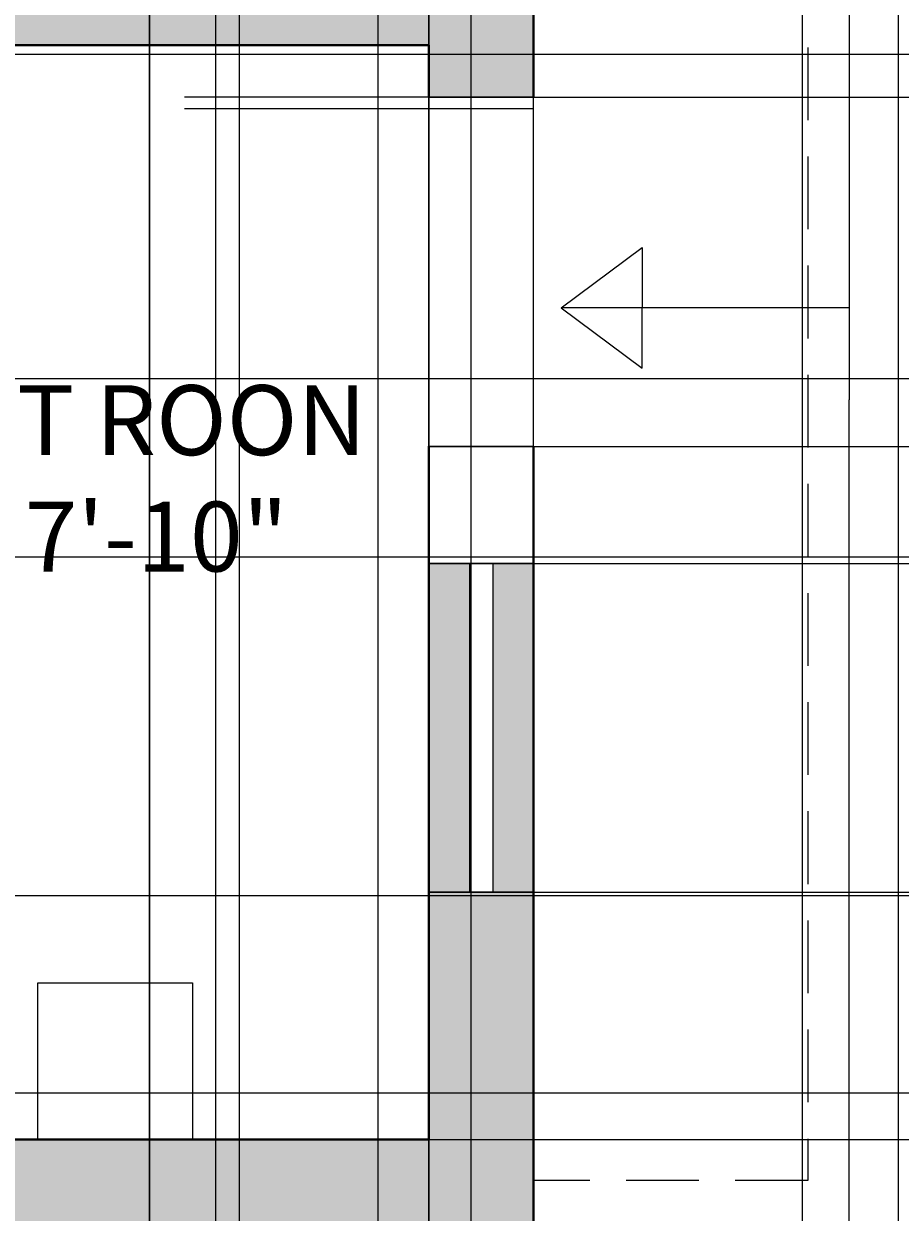
# Model space of a CAD drawing. Units: inches. Extents: x 818 to 1898, y 976 to 2364.
# Tile 53 of 96: x 1671 to 1746, y 1690 to 1792. Entities that reach past the tile are written whole.
import ezdxf

# ---------------------------------------------------------------- set-up
doc = ezdxf.new("R2010")
doc.units = ezdxf.units.IN
doc.header["$LTSCALE"] = 5
doc.header["$MEASUREMENT"] = 0
doc.linetypes.add('HIDDEN', pattern=[0.375, 0.25, -0.125])
for name, color, linetype, lineweight in [('A-ANNO-DIMS', 2, 'Continuous', 18), ('A-ANNO-SYMB', 7, 'Continuous', 18), ('A-AREA-IDEN', 7, 'Continuous', 18), ('A-DOOR', 3, 'Continuous', 25), ('A-FLOR-OVHD', 8, 'HIDDEN', 13), ('A-FLOR-STRS', 7, 'Continuous', 25), ('A-FURN', 8, 'Continuous', 18), ('A-GLAZ', 4, 'Continuous', 18), ('A-WALL', 7, 'Continuous', 40)]:
    doc.layers.add(name, color=color, linetype=linetype, lineweight=lineweight)
doc.layers.add('A-GLAZ-PATT', color=141, linetype='Continuous', lineweight=9, true_color=0xadddf7)
doc.layers.add('A-WALL-PATT', color=251, linetype='Continuous', lineweight=13, true_color=0x636466)
doc.styles.get("Standard").update_dxf_attribs({"font": 'arial.ttf'})
doc.dimstyles.get("Standard").update_dxf_attribs({"dimtxt": 0.18, "dimasz": 0.18, "dimexe": 0.18, "dimexo": 0.0625, "dimgap": 0.09, "dimtad": 0, "dimtih": 1, "dimtoh": 1, "dimdec": 4, "dimzin": 0, "dimdsep": 46, "dimtxsty": 'Standard', "dimcen": 0.09, "dimadec": 0, "dimazin": 0, "dimtfac": 1, "dimtdec": 4, "dimtofl": 0, "dimtmove": 0, "dimatfit": 3, "dimfxl": 1, "dimtolj": 1, "dimtzin": 0, "dimarcsym": 0})

# ---------------------------------------------------------------- blocks, each defined once
blk = doc.blocks.new('ARROW-STEP-UP')
at = {"ltscale": 5}
for p, q in [((0, 5.17), (6.97, 10.34)), ((6.97, 10.34), (6.97, 5.17)), ((24.75, 5.17), (0, 5.17)), ((0, 5.17), (6.97, 0)), ((6.97, 0), (6.97, 5.17))]:
    blk.add_line(p, q, dxfattribs=at)
blk = doc.blocks.new('*D71')
at = {"layer": 'A-ANNO-DIMS', "color": 0, "lineweight": -2, "ltscale": 5, "transparency": 16777216}
for p, q in [((1714.79, 2053.08), (1897.92, 2053.08)), ((1897.74, 2052.9), (1897.74, 1699.76)), ((1897.74, 1346.26), (1897.74, 1699.4)), ((1714.79, 1346.08), (1897.92, 1346.08))]:
    blk.add_line(p, q, dxfattribs=at)
at = {"layer": 'A-ANNO-DIMS', "color": 0, "ltscale": 5, "transparency": 16777216}
for points in [[(1897.71, 2052.9), (1897.77, 2052.9), (1897.74, 2053.08)], [(1897.71, 1346.26), (1897.77, 1346.26), (1897.74, 1346.08)]]:
    blk.add_solid(points, dxfattribs=at)
at = {"layer": 'Defpoints', "color": 0, "ltscale": 5, "transparency": 16777216}
for p in [(1714.73, 2053.08), (1897.74, 2053.08), (1714.73, 1346.08)]:
    blk.add_point(p, dxfattribs=at)
at = {"layer": 'A-ANNO-DIMS', "color": 0, "ltscale": 5, "transparency": 16777216, "insert": (1897.74, 1699.58), "char_height": 0.18, "attachment_point": 5}
blk.add_mtext('\\A1;707', dxfattribs=at)
blk = doc.blocks.new('*D75')
at = {"layer": 'A-ANNO-DIMS', "color": 0, "lineweight": -2, "ltscale": 5, "transparency": 16777216}
for p, q in [((1705.79, 1785.61), (1897.92, 1785.61)), ((1897.74, 1785.43), (1897.74, 1770.79)), ((1897.74, 1755.79), (1897.74, 1770.43)), ((1705.79, 1755.61), (1897.92, 1755.61))]:
    blk.add_line(p, q, dxfattribs=at)
at = {"layer": 'A-ANNO-DIMS', "color": 0, "ltscale": 5, "transparency": 16777216}
for points in [[(1897.71, 1785.43), (1897.77, 1785.43), (1897.74, 1785.61)], [(1897.71, 1755.79), (1897.77, 1755.79), (1897.74, 1755.61)]]:
    blk.add_solid(points, dxfattribs=at)
at = {"layer": 'Defpoints', "color": 0, "ltscale": 5, "transparency": 16777216}
for p in [(1705.73, 1785.61), (1705.73, 1755.61), (1897.74, 1755.61)]:
    blk.add_point(p, dxfattribs=at)
at = {"layer": 'A-ANNO-DIMS', "color": 0, "ltscale": 5, "transparency": 16777216, "insert": (1897.74, 1770.61), "char_height": 0.18, "attachment_point": 5}
blk.add_mtext('\\A1;30', dxfattribs=at)
blk = doc.blocks.new('*D85')
at = {"layer": 'A-ANNO-DIMS', "color": 0, "lineweight": -2, "ltscale": 5, "transparency": 16777216}
for p, q in [((1258.79, 2053.08), (1897.92, 2053.08)), ((1897.74, 2052.9), (1897.74, 1876.76)), ((1897.74, 1700.26), (1897.74, 1876.4)), ((1258.79, 1700.08), (1897.92, 1700.08))]:
    blk.add_line(p, q, dxfattribs=at)
at = {"layer": 'A-ANNO-DIMS', "color": 0, "ltscale": 5, "transparency": 16777216}
for points in [[(1897.71, 2052.9), (1897.77, 2052.9), (1897.74, 2053.08)], [(1897.71, 1700.26), (1897.77, 1700.26), (1897.74, 1700.08)]]:
    blk.add_solid(points, dxfattribs=at)
at = {"layer": 'Defpoints', "color": 0, "ltscale": 5, "transparency": 16777216}
for p in [(1258.73, 2053.08), (1897.74, 2053.08), (1258.73, 1700.08)]:
    blk.add_point(p, dxfattribs=at)
at = {"layer": 'A-ANNO-DIMS', "color": 0, "ltscale": 5, "transparency": 16777216, "insert": (1897.74, 1876.58), "char_height": 0.18, "attachment_point": 5}
blk.add_mtext('\\A1;353', dxfattribs=at)
blk = doc.blocks.new('*D103')
at = {"layer": 'A-ANNO-DIMS', "color": 0, "lineweight": -2, "ltscale": 5, "transparency": 16777216}
for p, q in [((1626.57, 1071.12), (1626.57, 2363.87)), ((1626.75, 2363.69), (1657.7, 2363.69)), ((1689.29, 2363.69), (1658.35, 2363.69)), ((1689.47, 1071.12), (1689.47, 2363.87))]:
    blk.add_line(p, q, dxfattribs=at)
at = {"layer": 'A-ANNO-DIMS', "color": 0, "ltscale": 5, "transparency": 16777216}
for points in [[(1626.75, 2363.72), (1626.75, 2363.66), (1626.57, 2363.69)], [(1689.29, 2363.72), (1689.29, 2363.66), (1689.47, 2363.69)]]:
    blk.add_solid(points, dxfattribs=at)
at = {"layer": 'Defpoints', "color": 0, "ltscale": 5, "transparency": 16777216}
for p in [(1689.47, 2363.69), (1626.57, 1071.06), (1689.47, 1071.06)]:
    blk.add_point(p, dxfattribs=at)
at = {"layer": 'A-ANNO-DIMS', "color": 0, "ltscale": 5, "transparency": 16777216, "insert": (1658.02, 2363.69), "char_height": 0.18, "attachment_point": 5}
blk.add_mtext('\\A1;62.9', dxfattribs=at)
blk = doc.blocks.new('*D104')
at = {"layer": 'A-ANNO-DIMS', "color": 0, "lineweight": -2, "ltscale": 5, "transparency": 16777216}
for p, q in [((1689.47, 1071.12), (1689.47, 2363.87)), ((1689.65, 2363.69), (1717.4, 2363.69)), ((1745.9, 2363.69), (1718.15, 2363.69)), ((1746.08, 1071.12), (1746.08, 2363.87))]:
    blk.add_line(p, q, dxfattribs=at)
at = {"layer": 'A-ANNO-DIMS', "color": 0, "ltscale": 5, "transparency": 16777216}
for points in [[(1689.65, 2363.72), (1689.65, 2363.66), (1689.47, 2363.69)], [(1745.9, 2363.72), (1745.9, 2363.66), (1746.08, 2363.69)]]:
    blk.add_solid(points, dxfattribs=at)
at = {"layer": 'Defpoints', "color": 0, "ltscale": 5, "transparency": 16777216}
for p in [(1746.08, 2363.69), (1689.47, 1071.06), (1746.08, 1071.06)]:
    blk.add_point(p, dxfattribs=at)
at = {"layer": 'A-ANNO-DIMS', "color": 0, "ltscale": 5, "transparency": 16777216, "insert": (1717.78, 2363.69), "char_height": 0.18, "attachment_point": 5}
blk.add_mtext('\\A1;56.61', dxfattribs=at)
blk = doc.blocks.new('*D119')
at = {"layer": 'A-ANNO-DIMS', "color": 0, "lineweight": -2, "ltscale": 5, "transparency": 16777216}
for p, q in [((1766.29, 1716.99), (818.03, 1716.99)), ((818.21, 1716.81), (818.21, 1672.43)), ((818.21, 1627.69), (818.21, 1672.06)), ((1766.29, 1627.51), (818.03, 1627.51))]:
    blk.add_line(p, q, dxfattribs=at)
at = {"layer": 'A-ANNO-DIMS', "color": 0, "ltscale": 5, "transparency": 16777216}
for points in [[(818.18, 1716.81), (818.24, 1716.81), (818.21, 1716.99)], [(818.18, 1627.69), (818.24, 1627.69), (818.21, 1627.51)]]:
    blk.add_solid(points, dxfattribs=at)
at = {"layer": 'Defpoints', "color": 0, "ltscale": 5, "transparency": 16777216}
for p in [(818.21, 1716.99), (1766.35, 1716.99), (1766.35, 1627.51)]:
    blk.add_point(p, dxfattribs=at)
at = {"layer": 'A-ANNO-DIMS', "color": 0, "ltscale": 5, "transparency": 16777216, "insert": (818.21, 1672.25), "char_height": 0.18, "attachment_point": 5}
blk.add_mtext('\\A1;89.48', dxfattribs=at)
blk = doc.blocks.new('*D120')
at = {"layer": 'A-ANNO-DIMS', "color": 0, "lineweight": -2, "ltscale": 5, "transparency": 16777216}
for p, q in [((1766.29, 1797.72), (818.03, 1797.72)), ((818.21, 1797.54), (818.21, 1757.53)), ((818.21, 1717.17), (818.21, 1757.17)), ((1766.29, 1716.99), (818.03, 1716.99))]:
    blk.add_line(p, q, dxfattribs=at)
at = {"layer": 'A-ANNO-DIMS', "color": 0, "ltscale": 5, "transparency": 16777216}
for points in [[(818.18, 1797.54), (818.24, 1797.54), (818.21, 1797.72)], [(818.18, 1717.17), (818.24, 1717.17), (818.21, 1716.99)]]:
    blk.add_solid(points, dxfattribs=at)
at = {"layer": 'Defpoints', "color": 0, "ltscale": 5, "transparency": 16777216}
for p in [(818.21, 1797.72), (1766.35, 1797.72), (1766.35, 1716.99)]:
    blk.add_point(p, dxfattribs=at)
at = {"layer": 'A-ANNO-DIMS', "color": 0, "ltscale": 5, "transparency": 16777216, "insert": (818.21, 1757.35), "char_height": 0.18, "attachment_point": 5}
blk.add_mtext('\\A1;80.73', dxfattribs=at)
blk = doc.blocks.new('*D154')
at = {"layer": 'A-ANNO-DIMS', "color": 0, "lineweight": -2, "ltscale": 5, "transparency": 16777216}
for p, q in [((1701.37, 1290.14), (1701.37, 2363.87)), ((1701.55, 2363.69), (1705.22, 2363.69)), ((1709.19, 2363.69), (1705.52, 2363.69)), ((1709.37, 1298.14), (1709.37, 2363.87))]:
    blk.add_line(p, q, dxfattribs=at)
at = {"layer": 'A-ANNO-DIMS', "color": 0, "ltscale": 5, "transparency": 16777216}
for points in [[(1701.55, 2363.72), (1701.55, 2363.66), (1701.37, 2363.69)], [(1709.19, 2363.72), (1709.19, 2363.66), (1709.37, 2363.69)]]:
    blk.add_solid(points, dxfattribs=at)
at = {"layer": 'Defpoints', "color": 0, "ltscale": 5, "transparency": 16777216}
for p in [(1709.37, 2363.69), (1709.37, 1298.08), (1701.37, 1290.08)]:
    blk.add_point(p, dxfattribs=at)
at = {"layer": 'A-ANNO-DIMS', "color": 0, "ltscale": 5, "transparency": 16777216, "insert": (1705.37, 2363.69), "char_height": 0.18, "attachment_point": 5}
blk.add_mtext('\\A1;8', dxfattribs=at)
blk = doc.blocks.new('*D186')
at = {"layer": 'A-ANNO-DIMS', "color": 0, "lineweight": -2, "ltscale": 5, "transparency": 16777216}
for p, q in [((1714.73, 1549.14), (1714.73, 2363.87)), ((1714.91, 2363.69), (1725.82, 2363.69)), ((1737.66, 2363.69), (1726.75, 2363.69)), ((1737.84, 1549.14), (1737.84, 2363.87))]:
    blk.add_line(p, q, dxfattribs=at)
at = {"layer": 'A-ANNO-DIMS', "color": 0, "ltscale": 5, "transparency": 16777216}
for points in [[(1714.91, 2363.72), (1714.91, 2363.66), (1714.73, 2363.69)], [(1737.66, 2363.72), (1737.66, 2363.66), (1737.84, 2363.69)]]:
    blk.add_solid(points, dxfattribs=at)
at = {"layer": 'Defpoints', "color": 0, "ltscale": 5, "transparency": 16777216}
for p in [(1737.84, 2363.69), (1714.73, 1549.08), (1737.84, 1549.08)]:
    blk.add_point(p, dxfattribs=at)
at = {"layer": 'A-ANNO-DIMS', "color": 0, "ltscale": 5, "transparency": 16777216, "insert": (1726.28, 2363.69), "char_height": 0.18, "attachment_point": 5}
blk.add_mtext('\\A1;23.116', dxfattribs=at)
blk = doc.blocks.new('*D195')
at = {"layer": 'A-ANNO-DIMS', "color": 0, "lineweight": -2, "ltscale": 5, "transparency": 16777216}
for p, q in [((1681.73, 1379.14), (1681.73, 2363.87)), ((1681.91, 2363.69), (1693.51, 2363.69)), ((1705.55, 2363.69), (1693.95, 2363.69)), ((1705.73, 1355.14), (1705.73, 2363.87))]:
    blk.add_line(p, q, dxfattribs=at)
at = {"layer": 'A-ANNO-DIMS', "color": 0, "ltscale": 5, "transparency": 16777216}
for points in [[(1681.91, 2363.72), (1681.91, 2363.66), (1681.73, 2363.69)], [(1705.55, 2363.72), (1705.55, 2363.66), (1705.73, 2363.69)]]:
    blk.add_solid(points, dxfattribs=at)
at = {"layer": 'Defpoints', "color": 0, "ltscale": 5, "transparency": 16777216}
for p in [(1705.73, 2363.69), (1681.73, 1379.08), (1705.73, 1355.08)]:
    blk.add_point(p, dxfattribs=at)
at = {"layer": 'A-ANNO-DIMS', "color": 0, "ltscale": 5, "transparency": 16777216, "insert": (1693.73, 2363.69), "char_height": 0.18, "attachment_point": 5}
blk.add_mtext('\\A1;24', dxfattribs=at)
blk = doc.blocks.new('*D212')
at = {"layer": 'A-ANNO-DIMS', "color": 0, "lineweight": -2, "ltscale": 5, "transparency": 16777216}
for p, q in [((1681.73, 1900.02), (1681.73, 975.66)), ((1705.73, 1876.02), (1705.73, 975.66)), ((1681.91, 975.84), (1693.51, 975.84)), ((1705.55, 975.84), (1693.95, 975.84))]:
    blk.add_line(p, q, dxfattribs=at)
at = {"layer": 'A-ANNO-DIMS', "color": 0, "ltscale": 5, "transparency": 16777216}
for points in [[(1681.91, 975.87), (1681.91, 975.81), (1681.73, 975.84)], [(1705.55, 975.87), (1705.55, 975.81), (1705.73, 975.84)]]:
    blk.add_solid(points, dxfattribs=at)
at = {"layer": 'Defpoints', "color": 0, "ltscale": 5, "transparency": 16777216}
for p in [(1681.73, 1900.08), (1705.73, 1876.08), (1705.73, 975.84)]:
    blk.add_point(p, dxfattribs=at)
at = {"layer": 'A-ANNO-DIMS', "color": 0, "ltscale": 5, "transparency": 16777216, "insert": (1693.73, 975.84), "char_height": 0.18, "attachment_point": 5}
blk.add_mtext('\\A1;24', dxfattribs=at)
blk = doc.blocks.new('*D216')
at = {"layer": 'A-ANNO-DIMS', "color": 0, "lineweight": -2, "ltscale": 5, "transparency": 16777216}
for p, q in [((1705.79, 1717.32), (1897.92, 1717.32)), ((1897.74, 1717.14), (1897.74, 1706.88)), ((1897.74, 1696.26), (1897.74, 1706.52)), ((1705.79, 1696.08), (1897.92, 1696.08))]:
    blk.add_line(p, q, dxfattribs=at)
at = {"layer": 'A-ANNO-DIMS', "color": 0, "ltscale": 5, "transparency": 16777216}
for points in [[(1897.71, 1717.14), (1897.77, 1717.14), (1897.74, 1717.32)], [(1897.71, 1696.26), (1897.77, 1696.26), (1897.74, 1696.08)]]:
    blk.add_solid(points, dxfattribs=at)
at = {"layer": 'Defpoints', "color": 0, "ltscale": 5, "transparency": 16777216}
for p in [(1705.73, 1717.32), (1897.74, 1717.32), (1705.73, 1696.08)]:
    blk.add_point(p, dxfattribs=at)
at = {"layer": 'A-ANNO-DIMS', "color": 0, "ltscale": 5, "transparency": 16777216, "insert": (1897.74, 1706.7), "char_height": 0.18, "attachment_point": 5}
blk.add_mtext('\\A1;21.24', dxfattribs=at)
blk = doc.blocks.new('*D217')
at = {"layer": 'A-ANNO-DIMS', "color": 0, "lineweight": -2, "ltscale": 5, "transparency": 16777216}
for p, q in [((1705.79, 1745.56), (1897.92, 1745.56)), ((1897.74, 1745.38), (1897.74, 1731.62)), ((1897.74, 1717.5), (1897.74, 1731.26)), ((1705.79, 1717.32), (1897.92, 1717.32))]:
    blk.add_line(p, q, dxfattribs=at)
at = {"layer": 'A-ANNO-DIMS', "color": 0, "ltscale": 5, "transparency": 16777216}
for points in [[(1897.71, 1745.38), (1897.77, 1745.38), (1897.74, 1745.56)], [(1897.71, 1717.5), (1897.77, 1717.5), (1897.74, 1717.32)]]:
    blk.add_solid(points, dxfattribs=at)
at = {"layer": 'Defpoints', "color": 0, "ltscale": 5, "transparency": 16777216}
for p in [(1705.73, 1745.56), (1897.74, 1745.56), (1705.73, 1717.32)]:
    blk.add_point(p, dxfattribs=at)
at = {"layer": 'A-ANNO-DIMS', "color": 0, "ltscale": 5, "transparency": 16777216, "insert": (1897.74, 1731.44), "char_height": 0.18, "attachment_point": 5}
blk.add_mtext('\\A1;28.24', dxfattribs=at)
blk = doc.blocks.new('*D221')
at = {"layer": 'A-ANNO-DIMS', "color": 0, "lineweight": -2, "ltscale": 5, "transparency": 16777216}
for p, q in [((1668.18, 1696.02), (1668.18, 975.66)), ((1705.73, 1696.02), (1705.73, 975.66)), ((1668.36, 975.84), (1686.56, 975.84)), ((1705.55, 975.84), (1687.35, 975.84))]:
    blk.add_line(p, q, dxfattribs=at)
at = {"layer": 'A-ANNO-DIMS', "color": 0, "ltscale": 5, "transparency": 16777216}
for points in [[(1668.36, 975.87), (1668.36, 975.81), (1668.18, 975.84)], [(1705.55, 975.87), (1705.55, 975.81), (1705.73, 975.84)]]:
    blk.add_solid(points, dxfattribs=at)
at = {"layer": 'Defpoints', "color": 0, "ltscale": 5, "transparency": 16777216}
for p in [(1668.18, 1696.08), (1705.73, 1696.08), (1705.73, 975.84)]:
    blk.add_point(p, dxfattribs=at)
at = {"layer": 'A-ANNO-DIMS', "color": 0, "ltscale": 5, "transparency": 16777216, "insert": (1686.95, 975.84), "char_height": 0.18, "attachment_point": 5}
blk.add_mtext('\\A1;37.54', dxfattribs=at)
blk = doc.blocks.new('*D228')
at = {"layer": 'A-ANNO-DIMS', "color": 0, "lineweight": -2, "ltscale": 5, "transparency": 16777216}
for p, q in [((1687.39, 1802.02), (1687.39, 975.66)), ((1705.73, 1802.02), (1705.73, 975.66)), ((1687.57, 975.84), (1696.17, 975.84)), ((1705.55, 975.84), (1696.94, 975.84))]:
    blk.add_line(p, q, dxfattribs=at)
at = {"layer": 'A-ANNO-DIMS', "color": 0, "ltscale": 5, "transparency": 16777216}
for points in [[(1687.57, 975.87), (1687.57, 975.81), (1687.39, 975.84)], [(1705.55, 975.87), (1705.55, 975.81), (1705.73, 975.84)]]:
    blk.add_solid(points, dxfattribs=at)
at = {"layer": 'Defpoints', "color": 0, "ltscale": 5, "transparency": 16777216}
for p in [(1687.39, 1802.08), (1705.73, 1802.08), (1705.73, 975.84)]:
    blk.add_point(p, dxfattribs=at)
at = {"layer": 'A-ANNO-DIMS', "color": 0, "ltscale": 5, "transparency": 16777216, "insert": (1696.56, 975.84), "char_height": 0.18, "attachment_point": 5}
blk.add_mtext('\\A1;18.33', dxfattribs=at)
blk = doc.blocks.new('*D268')
at = {"layer": 'A-ANNO-DIMS', "color": 0, "lineweight": -2, "ltscale": 5, "transparency": 16777216}
for p, q in [((1741.9, 1890.29), (1897.92, 1890.29)), ((1897.74, 1890.11), (1897.74, 1788.87)), ((1897.74, 1687.26), (1897.74, 1788.5)), ((1741.9, 1687.08), (1897.92, 1687.08))]:
    blk.add_line(p, q, dxfattribs=at)
at = {"layer": 'A-ANNO-DIMS', "color": 0, "ltscale": 5, "transparency": 16777216}
for points in [[(1897.71, 1890.11), (1897.77, 1890.11), (1897.74, 1890.29)], [(1897.71, 1687.26), (1897.77, 1687.26), (1897.74, 1687.08)]]:
    blk.add_solid(points, dxfattribs=at)
at = {"layer": 'Defpoints', "color": 0, "ltscale": 5, "transparency": 16777216}
for p in [(1741.84, 1890.29), (1897.74, 1890.29), (1741.84, 1687.08)]:
    blk.add_point(p, dxfattribs=at)
at = {"layer": 'A-ANNO-DIMS', "color": 0, "ltscale": 5, "transparency": 16777216, "insert": (1897.74, 1788.68), "char_height": 0.18, "attachment_point": 5}
blk.add_mtext('\\A1;203.2', dxfattribs=at)
blk = doc.blocks.new('*D280')
at = {"layer": 'A-ANNO-DIMS', "color": 0, "lineweight": -2, "ltscale": 5, "transparency": 16777216}
for p, q in [((1398.73, 1789.31), (1897.92, 1789.31)), ((1897.74, 1789.13), (1897.74, 1767.89)), ((1897.74, 1746.29), (1897.74, 1767.53)), ((1397.41, 1746.11), (1897.92, 1746.11))]:
    blk.add_line(p, q, dxfattribs=at)
at = {"layer": 'A-ANNO-DIMS', "color": 0, "ltscale": 5, "transparency": 16777216}
for points in [[(1897.71, 1789.13), (1897.77, 1789.13), (1897.74, 1789.31)], [(1897.71, 1746.29), (1897.77, 1746.29), (1897.74, 1746.11)]]:
    blk.add_solid(points, dxfattribs=at)
at = {"layer": 'Defpoints', "color": 0, "ltscale": 5, "transparency": 16777216}
for p in [(1398.67, 1789.31), (1897.74, 1789.31), (1397.35, 1746.11)]:
    blk.add_point(p, dxfattribs=at)
at = {"layer": 'A-ANNO-DIMS', "color": 0, "ltscale": 5, "transparency": 16777216, "insert": (1897.74, 1767.71), "char_height": 0.18, "attachment_point": 5}
blk.add_mtext('\\A1;43.19', dxfattribs=at)
blk = doc.blocks.new('*D282')
at = {"layer": 'A-ANNO-DIMS', "color": 0, "lineweight": -2, "ltscale": 5, "transparency": 16777216}
for p, q in [((1422.08, 2081.19), (1897.92, 2081.19)), ((1897.74, 2081.01), (1897.74, 1884.32)), ((1897.74, 1687.26), (1897.74, 1883.95)), ((1463.79, 1687.08), (1897.92, 1687.08))]:
    blk.add_line(p, q, dxfattribs=at)
at = {"layer": 'A-ANNO-DIMS', "color": 0, "ltscale": 5, "transparency": 16777216}
for points in [[(1897.71, 2081.01), (1897.77, 2081.01), (1897.74, 2081.19)], [(1897.71, 1687.26), (1897.77, 1687.26), (1897.74, 1687.08)]]:
    blk.add_solid(points, dxfattribs=at)
at = {"layer": 'Defpoints', "color": 0, "ltscale": 5, "transparency": 16777216}
for p in [(1422.02, 2081.19), (1897.74, 2081.19), (1463.73, 1687.08)]:
    blk.add_point(p, dxfattribs=at)
at = {"layer": 'A-ANNO-DIMS', "color": 0, "ltscale": 5, "transparency": 16777216, "insert": (1897.74, 1884.13), "char_height": 0.18, "attachment_point": 5}
blk.add_mtext('\\A1;394.1', dxfattribs=at)
blk = doc.blocks.new('*D284')
at = {"layer": 'A-ANNO-DIMS', "color": 0, "lineweight": -2, "ltscale": 5, "transparency": 16777216}
for p, q in [((1351.66, 1761.45), (1897.92, 1761.45)), ((1897.74, 1761.27), (1897.74, 1728.95)), ((1897.74, 1696.26), (1897.74, 1728.58)), ((1267.79, 1696.08), (1897.92, 1696.08))]:
    blk.add_line(p, q, dxfattribs=at)
at = {"layer": 'A-ANNO-DIMS', "color": 0, "ltscale": 5, "transparency": 16777216}
for points in [[(1897.71, 1761.27), (1897.77, 1761.27), (1897.74, 1761.45)], [(1897.71, 1696.26), (1897.77, 1696.26), (1897.74, 1696.08)]]:
    blk.add_solid(points, dxfattribs=at)
at = {"layer": 'Defpoints', "color": 0, "ltscale": 5, "transparency": 16777216}
for p in [(1351.6, 1761.45), (1267.73, 1696.08), (1897.74, 1696.08)]:
    blk.add_point(p, dxfattribs=at)
at = {"layer": 'A-ANNO-DIMS', "color": 0, "ltscale": 5, "transparency": 16777216, "insert": (1897.74, 1728.76), "char_height": 0.18, "attachment_point": 5}
blk.add_mtext('\\A1;65.37', dxfattribs=at)

msp = doc.modelspace()

# ---------------------------------------------------------------- hatches: boundary and pattern name
at = {"layer": 'A-GLAZ-PATT', "ltscale": 5}
h = msp.add_hatch(color=256, dxfattribs=at)
h.dxf.hatch_style = 1
h.paths.add_polyline_path([(1283.8183, 1504.5782), (1206.7252, 1504.5782), (1206.7252, 1501.0782), (1283.8183, 1501.0782)])
h.paths.add_polyline_path([(1283.8183, 1510.0782), (1206.7252, 1510.0782), (1206.7252, 1506.5782), (1283.8183, 1506.5782)])
h.paths.add_polyline_path([(1490.9163, 1355.0782), (1439.7252, 1355.0782), (1439.7252, 1409.0522), (1436.2252, 1409.0522), (1436.2252, 1351.5782), (1490.9163, 1351.5782)])
h.paths.add_polyline_path([(1434.2252, 1409.0522), (1430.7252, 1409.0522), (1430.7252, 1346.0782), (1435.0799, 1346.0782), (1435.0731, 1346.1152), (1435.1501, 1346.0782), (1490.9163, 1346.0782), (1490.9163, 1349.5782), (1434.2252, 1349.5782)])
h.paths.add_polyline_path([(1714.7251, 1545.0782), (1711.2252, 1545.0782), (1711.2252, 1521.0782), (1714.7251, 1521.0782)])
h.paths.add_polyline_path([(1709.2252, 1545.0782), (1705.7251, 1545.0782), (1705.7251, 1521.0782), (1709.2252, 1521.0782)])
h.paths.add_polyline_path([(1714.7251, 1687.0782), (1711.2252, 1687.0782), (1711.2252, 1649.9029), (1714.7251, 1649.9029)])
h.paths.add_polyline_path([(1709.2252, 1687.0782), (1705.7251, 1687.0782), (1705.7251, 1649.9029), (1709.2252, 1649.9029)])
h.paths.add_polyline_path([(1709.2252, 1745.5584), (1705.7251, 1745.5584), (1705.7251, 1717.3178), (1709.2252, 1717.3178)])
h.paths.add_polyline_path([(1714.7251, 1745.5584), (1711.2252, 1745.5584), (1711.2252, 1717.3178), (1714.7251, 1717.3178)])
h.paths.add_polyline_path([(1714.7251, 2014.5114), (1711.2252, 2014.5114), (1711.2252, 1962.0338), (1714.7251, 1962.0338)])
h.paths.add_polyline_path([(1709.2252, 2014.5114), (1705.7251, 2014.5114), (1705.7251, 1962.0338), (1709.2252, 1962.0338)])
h.paths.add_polyline_path([(1538.5155, 2047.5782), (1485.1216, 2047.5782), (1485.1216, 2044.0782), (1538.5155, 2044.0782)])
h.paths.add_polyline_path([(1538.5155, 2053.0782), (1485.1216, 2053.0782), (1485.1216, 2049.5782), (1538.5155, 2049.5782)])
h.paths.add_polyline_path([(1388.0315, 2047.5782), (1330.305, 2047.5782), (1330.305, 2044.0782), (1388.0315, 2044.0782)])
h.paths.add_polyline_path([(1388.0315, 2053.0782), (1330.305, 2053.0782), (1330.305, 2049.5782), (1388.0315, 2049.5782)])
h.paths.add_polyline_path([(1262.2252, 2019.2871), (1258.7251, 2019.2871), (1258.7251, 1928.9218), (1262.2252, 1928.9218)])
h.paths.add_polyline_path([(1267.7251, 2019.2871), (1264.2252, 2019.2871), (1264.2252, 1928.9218), (1267.7251, 1928.9218)])
h.paths.add_polyline_path([(1262.2252, 1862.9652), (1258.7251, 1862.9652), (1258.7251, 1814.9652), (1262.2252, 1814.9652)])
h.paths.add_polyline_path([(1267.7251, 1862.9652), (1264.2252, 1862.9652), (1264.2252, 1814.9652), (1267.7251, 1814.9652)])
h.paths.add_polyline_path([(1262.2252, 1755.3321), (1258.7251, 1755.3321), (1258.7251, 1707.3321), (1262.2252, 1707.3321)])
h.paths.add_polyline_path([(1267.7251, 1755.3321), (1264.2252, 1755.3321), (1264.2252, 1707.3321), (1267.7251, 1707.3321)])
h.paths.add_polyline_path([(1251.9333, 1692.5782), (1206.7252, 1692.5782), (1206.7252, 1687.0782), (1251.9333, 1687.0782)])
h.paths.add_polyline_path([(1251.9333, 1700.0782), (1206.7252, 1700.0782), (1206.7252, 1694.5782), (1251.9333, 1694.5782)])
at = {"layer": 'A-WALL-PATT', "ltscale": 5}
h = msp.add_hatch(color=256, dxfattribs=at)
h.dxf.hatch_style = 1
h.paths.add_polyline_path([(1267.7251, 1928.9218), (1258.7251, 1928.9218), (1258.7251, 1913.6401), (1250.3029, 1913.6401), (1250.3029, 1878.3919), (1258.7251, 1878.3919), (1258.7251, 1862.9652), (1267.7251, 1862.9652)])
h.paths.add_polyline_path([(1267.7251, 1814.9652), (1258.7251, 1814.9652), (1258.7251, 1755.3321), (1267.7251, 1755.3321)])
h.paths.add_polyline_path([(1463.7251, 1696.0782), (1267.7251, 1696.0782), (1267.7251, 1707.3321), (1258.7251, 1707.3321), (1258.7251, 1700.0782), (1251.9333, 1700.0782), (1251.9333, 1687.0782), (1463.7251, 1687.0782)])
h.paths.add_polyline_path([(1714.7251, 1717.3178), (1705.7251, 1717.3178), (1705.7251, 1696.0782), (1599.7252, 1696.0782), (1599.7252, 1790.0782), (1705.7251, 1790.0782), (1705.7251, 1785.6125), (1714.7251, 1785.6125), (1714.7251, 1827.2125), (1705.7251, 1827.2125), (1705.7251, 1802.0782), (1599.7252, 1802.0782), (1599.7252, 1867.0782), (1705.7251, 1867.0782), (1705.7251, 1857.2125), (1714.7251, 1857.2125), (1714.7251, 1930.0316), (1741.8409, 1930.0316), (1741.8409, 1935.0316), (1714.7251, 1935.0316), (1714.7251, 1957.0338), (1741.8409, 1957.0338), (1741.8409, 1962.0338), (1714.7251, 1962.0338), (1705.7251, 1962.0338), (1705.7251, 1948.0782), (1599.7252, 1948.0782), (1599.7252, 1981.0782), (1590.7252, 1981.0782), (1590.7252, 1941.0782), (1620.7252, 1941.0782), (1705.7251, 1941.0782), (1705.7251, 1876.0782), (1599.7252, 1876.0782), (1599.7252, 1911.0782), (1590.7252, 1911.0782), (1590.7252, 1876.0782), (1429.2252, 1876.0782), (1429.2252, 1867.0782), (1511.7252, 1867.0782), (1528.593, 1867.0782), (1595.7252, 1867.0782), (1595.7252, 1773.0782), (1520.7252, 1773.0782), (1520.7252, 1837.5823), (1532.593, 1837.5823), (1532.593, 1867.0782), (1528.593, 1867.0782), (1528.593, 1841.5823), (1511.7252, 1841.5823), (1511.7252, 1744.9714), (1520.7252, 1744.9714), (1520.7252, 1761.0782), (1595.7252, 1761.0782), (1595.7252, 1696.0782), (1520.7252, 1696.0782), (1520.7252, 1716.0454), (1511.7252, 1716.0454), (1511.7252, 1696.0782), (1511.7252, 1687.0782), (1714.7251, 1687.0782)])
h.paths.add_polyline_path([(1714.7251, 2053.0782), (1714.7251, 2081.1881), (1709.7252, 2081.1881), (1709.7252, 2053.0782), (1681.6446, 2053.0782), (1681.6446, 2081.1881), (1676.6446, 2081.1881), (1676.6446, 2053.0782), (1538.5155, 2053.0782), (1538.5155, 2044.0782), (1590.7252, 2044.0782), (1590.7252, 2011.0782), (1599.7252, 2011.0782), (1599.7252, 2044.0782), (1705.7251, 2044.0782), (1705.7251, 2014.5114), (1714.7251, 2014.5114)])
h.paths.add_polyline_path([(1485.1216, 2053.0782), (1422.02, 2053.0782), (1422.02, 2081.1881), (1413.02, 2081.1881), (1413.02, 2053.0782), (1399.6356, 2053.0782), (1399.6356, 2081.1881), (1390.6356, 2081.1881), (1390.6356, 2053.0782), (1388.0315, 2053.0782), (1388.0315, 2044.0782), (1416.2743, 2044.0782), (1485.1216, 2044.0782)])
h.paths.add_polyline_path([(1330.305, 2053.0782), (1258.7251, 2053.0782), (1258.7251, 2019.2871), (1267.7251, 2019.2871), (1267.7251, 2044.0782), (1330.305, 2044.0782)])
h.paths.add_polyline_path([(1258.7251, 2053.0782), (1214.6577, 2053.0782), (1214.6577, 2044.0782), (1258.7251, 2044.0782)])
h.paths.add_polyline_path([(1214.6577, 2053.0782), (1180.349, 2053.0782), (1180.349, 2044.0782), (1214.6577, 2044.0782)])
h.paths.add_polyline_path([(1714.7251, 1639.5782), (1741.8409, 1639.5782), (1741.8409, 1643.5782), (1714.7251, 1643.5782), (1714.7251, 1649.9029), (1705.7251, 1649.9029), (1705.7251, 1600.0782), (1477.7252, 1600.0782), (1477.7252, 1591.0782), (1520.7252, 1591.0782), (1616.7252, 1591.0782), (1616.7252, 1416.6857), (1622.7252, 1416.6857), (1622.7252, 1463.0782), (1624.7252, 1463.0782), (1624.7252, 1467.0782), (1622.7252, 1467.0782), (1622.7252, 1591.0782), (1705.7251, 1591.0782), (1705.7251, 1545.0782), (1714.7251, 1545.0782), (1741.8409, 1545.0782), (1741.8409, 1549.0782), (1714.7251, 1549.0782), (1714.7251, 1593.9175), (1737.8409, 1593.9175), (1737.8409, 1597.9175), (1714.7251, 1597.9175)])
h.paths.add_polyline_path([(1674.9024, 2060.7419), (1714.7045, 2060.7419), (1714.7045, 2073.1061), (1674.9024, 2073.1061)], flags=25)
h.paths.add_polyline_path([(1394.5468, 2061.6618), (1422.2344, 2061.6618), (1422.2344, 2074.0261), (1394.5468, 2074.0261)], flags=24)

# ---------------------------------------------------------------- linework, layer by layer
at = {"layer": 'A-DOOR'}
for p, q in [((1714.7251, 1785.6125), (1684.7252, 1785.6125)), ((1705.7251, 1785.6125), (1714.7251, 1785.6125)), ((1714.7251, 1784.6125), (1684.7252, 1784.6125)), ((1705.7251, 1755.6125), (1714.7251, 1755.6125))]:
    msp.add_line(p, q, dxfattribs=at)
at = {"layer": 'A-FLOR-OVHD', "ltscale": 5}
for p, q in [((1738.3002, 1883.6351), (1738.3002, 1692.5441)), ((1738.3002, 1692.5441), (1714.7251, 1692.5441))]:
    msp.add_line(p, q, dxfattribs=at)
at = {"layer": 'A-FLOR-STRS'}
for p in [(1741.8409, 1890.2903), (1741.8409, 1687.0782)]:
    msp.add_line(p, (1741.8409, 1759.6099), dxfattribs=at)
at = {"layer": 'A-FURN'}
msp.add_lwpolyline([(1672.1245, 1709.5388), (1685.4205, 1709.5388), (1685.4205, 1696.0782), (1672.1245, 1696.0782)], close=True, dxfattribs=at)
at = {"layer": 'A-GLAZ'}
for p, q in [((1714.7251, 1745.5584), (1705.7251, 1745.5584)), ((1709.2252, 1745.5584), (1709.2252, 1717.3178)), ((1711.2252, 1745.5584), (1711.2252, 1717.3178)), ((1714.7251, 1717.3178), (1705.7251, 1717.3178))]:
    msp.add_line(p, q, dxfattribs=at)
at = {"layer": 'A-WALL'}
for p, q in [((1714.7251, 1827.2125), (1714.7251, 1785.6125)), ((1599.7252, 1790.0782), (1705.7251, 1790.0782)), ((1705.7251, 1790.0782), (1705.7251, 1785.6125)), ((1705.7251, 1755.6125), (1705.7251, 1696.0782)), ((1714.7251, 1755.6125), (1714.7251, 1643.5782)), ((1599.7252, 1696.0782), (1705.7251, 1696.0782))]:
    msp.add_line(p, q, dxfattribs=at)

# ---------------------------------------------------------------- block references
at = {"layer": 'A-ANNO-SYMB'}
msp.add_blockref('ARROW-STEP-UP', (1717.086, 1762.3387), dxfattribs=at)

# ---------------------------------------------------------------- texts
at = {"layer": 'A-AREA-IDEN', "ltscale": 5, "insert": (1640.016, 1760.8611), "char_height": 6, "attachment_point": 1}
msp.add_mtext_dynamic_manual_height_columns('SERVENT ROON\\P8\'-10" X 7\'-10"', width=118.992422, gutter_width=1, heights=[0], dxfattribs=at)

# ---------------------------------------------------------------- dimensions: what is measured, and where the dimension line sits
at = {"layer": 'A-ANNO-DIMS', "ltscale": 5}
for base, p1, p2, override, picture, middle in [((1689.4714, 2363.6929), (1626.5748, 1071.0552), (1689.4714, 1071.0552), {"dimdec": 1, "dimlfac": 1, "dimrnd": 0, "dimzin": 0, "dimdsep": 46, "dimlunit": 2}, '*D103', (1658.0231, 2363.6929)), ((1705.7251, 2363.6929), (1681.7251, 1379.0782), (1705.7251, 1355.0782), {"dimdec": 0, "dimlfac": 1, "dimrnd": 0, "dimzin": 0, "dimdsep": 46, "dimlunit": 2}, '*D195', (1693.7251, 2363.6929)), ((1746.0831, 2363.6929), (1689.4714, 1071.0552), (1746.0831, 1071.0552), {"dimdec": 2, "dimlfac": 1, "dimrnd": 0, "dimzin": 0, "dimdsep": 46, "dimlunit": 2}, '*D104', (1717.7772, 2363.6929)), ((1709.3688, 2363.6929), (1701.3688, 1290.0782), (1709.3688, 1298.0782), {"dimdec": 0, "dimlfac": 1, "dimrnd": 0, "dimzin": 0, "dimdsep": 46, "dimlunit": 2}, '*D154', (1705.3688, 2363.6929)), ((1737.8409, 2363.6929), (1714.7251, 1549.0782), (1737.8409, 1549.0782), {"dimdec": 3, "dimlfac": 1, "dimrnd": 0, "dimzin": 0, "dimdsep": 46, "dimlunit": 2}, '*D186', (1726.283, 2363.6929)), ((1705.7251, 975.8433), (1681.7251, 1900.0782), (1705.7251, 1876.0782), {"dimdec": 0, "dimlfac": 1, "dimrnd": 0, "dimzin": 0, "dimdsep": 46, "dimlunit": 2}, '*D212', (1693.7251, 975.8433)), ((1705.7251, 975.8433), (1687.394, 1802.0782), (1705.7251, 1802.0782), {"dimdec": 2, "dimlfac": 1, "dimrnd": 0, "dimzin": 0, "dimdsep": 46, "dimlunit": 2}, '*D228', (1696.5596, 975.8433)), ((1705.7251, 975.8433), (1668.1841, 1696.0782), (1705.7251, 1696.0782), {"dimdec": 2, "dimlfac": 1, "dimrnd": 0, "dimzin": 0, "dimdsep": 46, "dimlunit": 2}, '*D221', (1686.9546, 975.8433))]:
    dim = msp.add_linear_dim(base=base, p1=p1, p2=p2, dimstyle='Standard', override=override, dxfattribs=at)
    dim.commit()
    dim.dimension.update_dxf_attribs({"geometry": picture, "text_midpoint": middle})
for base, p1, p2, override, picture, middle in [((1897.736, 2081.1881), (1463.7251, 1687.0782), (1422.02, 2081.1881), {"dimdec": 1, "dimlfac": 1, "dimrnd": 0, "dimzin": 0, "dimdsep": 46, "dimlunit": 2}, '*D282', (1897.736, 1884.1332)), ((1897.736, 2053.0782), (1258.7251, 1700.0782), (1258.7251, 2053.0782), {"dimdec": 0, "dimlfac": 1, "dimrnd": 0, "dimzin": 0, "dimdsep": 46, "dimlunit": 2}, '*D85', (1897.736, 1876.5782)), ((1897.736, 2053.0782), (1714.7251, 1346.0782), (1714.7251, 2053.0782), {"dimdec": 0, "dimlfac": 1, "dimrnd": 0, "dimzin": 0, "dimdsep": 46, "dimlunit": 2}, '*D71', (1897.736, 1699.5782)), ((1897.736, 1890.2903), (1741.8409, 1687.0782), (1741.8409, 1890.2903), {"dimdec": 1, "dimlfac": 1, "dimrnd": 0, "dimzin": 0, "dimdsep": 46, "dimlunit": 2}, '*D268', (1897.736, 1788.6843)), ((818.2059, 1797.7165), (1766.3524, 1716.9866), (1766.3524, 1797.7165), {"dimdec": 2, "dimlfac": 1, "dimrnd": 0, "dimzin": 0, "dimdsep": 46, "dimlunit": 2}, '*D120', (818.2059, 1757.3516)), ((1897.736, 1789.3057), (1397.3459, 1746.1142), (1398.6717, 1789.3057), {"dimdec": 2, "dimlfac": 1, "dimrnd": 0, "dimzin": 0, "dimdsep": 46, "dimlunit": 2}, '*D280', (1897.736, 1767.71)), ((1897.736, 1755.6125), (1705.7251, 1785.6125), (1705.7251, 1755.6125), {"dimdec": 0, "dimlfac": 1, "dimrnd": 0, "dimzin": 0, "dimdsep": 46, "dimlunit": 2}, '*D75', (1897.736, 1770.6125)), ((1897.736, 1696.0782), (1351.5985, 1761.449), (1267.7251, 1696.0782), {"dimdec": 2, "dimlfac": 1, "dimrnd": 0, "dimzin": 0, "dimdsep": 46, "dimlunit": 2}, '*D284', (1897.736, 1728.7636)), ((1897.736, 1745.5584), (1705.7251, 1717.3178), (1705.7251, 1745.5584), {"dimdec": 2, "dimlfac": 1, "dimrnd": 0, "dimzin": 0, "dimdsep": 46, "dimlunit": 2}, '*D217', (1897.736, 1731.4381)), ((1897.736, 1717.3178), (1705.7251, 1696.0782), (1705.7251, 1717.3178), {"dimdec": 2, "dimlfac": 1, "dimrnd": 0, "dimzin": 0, "dimdsep": 46, "dimlunit": 2}, '*D216', (1897.736, 1706.698)), ((818.2059, 1716.9866), (1766.3524, 1627.5052), (1766.3524, 1716.9866), {"dimdec": 2, "dimlfac": 1, "dimrnd": 0, "dimzin": 0, "dimdsep": 46, "dimlunit": 2}, '*D119', (818.2059, 1672.2459))]:
    dim = msp.add_linear_dim(base=base, p1=p1, p2=p2, angle=90, dimstyle='Standard', override=override, dxfattribs=at)
    dim.commit()
    dim.dimension.update_dxf_attribs({"geometry": picture, "text_midpoint": middle})

doc.saveas('drawing.dxf')
